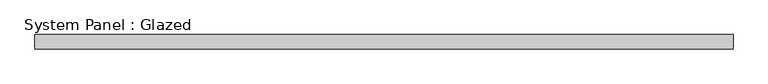
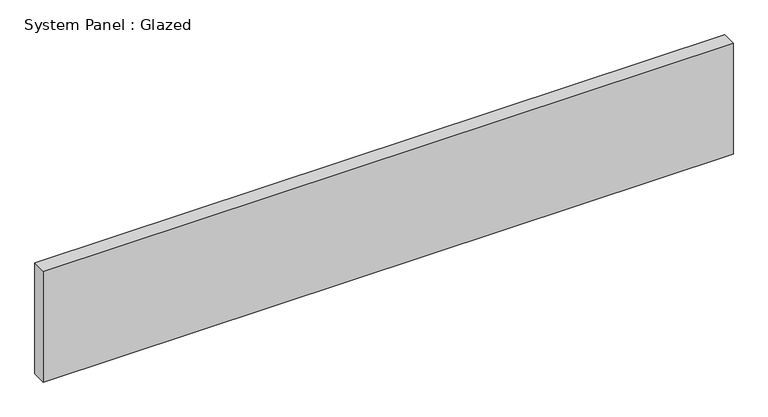
"""IFC4 building model written with IfcOpenShell, lengths in millimetres: plate geometry, System Panel : Glazed."""

from ifc_helpers import new_model, si_unit, origin, origin_with_axes, place, context, project, spatial, polyline, outline, extrude, source, transform, mapped, element, save


def system_panel_glazed_8059ee36(model_context):
    return source(origin(), model_context, "Body", "SweptSolid", [
        extrude(outline(polyline([(615.9499999, 19.05), (-615.9499999, 19.05), (-615.9499999, 44.45), (615.9499999, 44.45), (615.9499999, 19.05)])), origin_with_axes(), (0.0, 0.0, 1.0), 209.55),
    ])


if __name__ == "__main__":
    model = new_model("IFC4")
    model_context = context("Model", 3, world=origin())
    ifc_project = project(units=[si_unit("LENGTHUNIT", "METRE", prefix="MILLI")], contexts=[model_context])
    site = spatial("IfcSite", under=ifc_project)
    building = spatial("IfcBuilding", under=site)
    placement = place(None, origin())
    system_panel_glazed_shape = system_panel_glazed_8059ee36(model_context)
    element("IfcPlate", 1, ObjectType="System Panel : Glazed", at=placement, inside=building, context=model_context, shape_type="MappedRepresentation", body=[
        mapped(system_panel_glazed_shape, transform((0.0, 0.0, 0.0), x_axis=(1.0, 0.0, 0.0), y_axis=(0.0, 1.0, 0.0), z_axis=(0.0, 0.0, 1.0))),
    ])
    save(model, "model.ifc")

# Revit data of these elements
# Type "System Panel : Glazed"
#   Construction Type Id = "GSP4R"
#   Analytic Construction = "1/8 in Pilkington single glazing"
#   Visual Light Transmittance = 0.9
#   Solar Heat Gain Coefficient = 0.86
#   Heat Transfer Coefficient (U) = 1.18115 BTU/(h·ft²·°F)
#   Define Thermal Properties by = 1
# Element 1 (IfcPlate, "System Panel : Glazed")
#   Materials on its faces: "Glass"
# Materials
#   "Glass": class "Glass", colour RGB 0 128 192, transparency 0.75, Description = "Soda Lime Glass", Cost = 0
